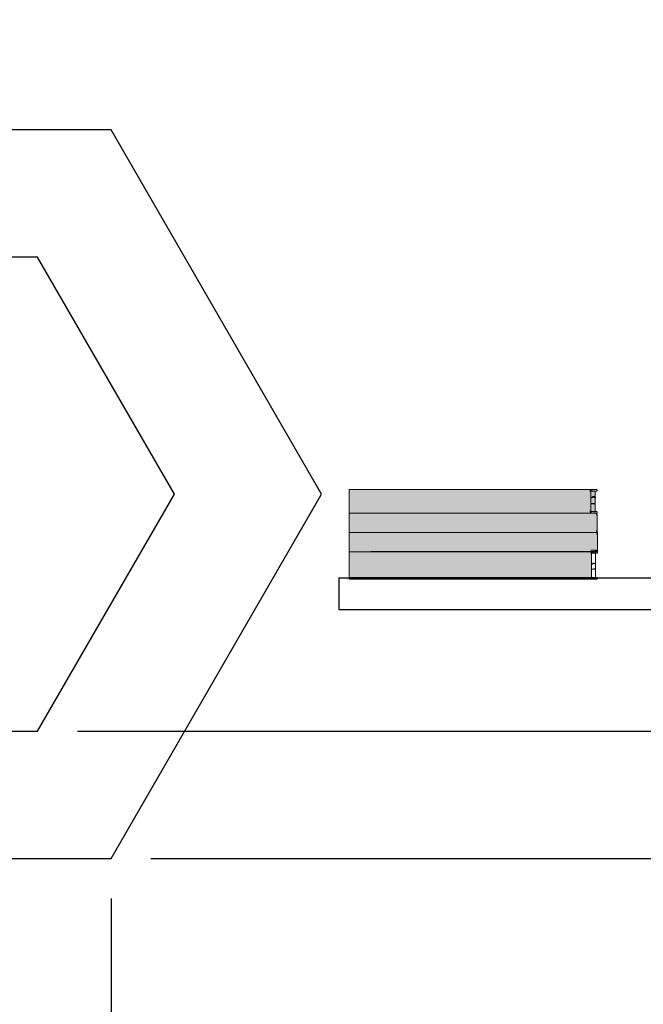
# Model space of a CAD drawing. Units: millimetres. Extents: x 7894 to 8038, y 6851 to 6951.
# Tile 24 of 49: x 7948.9 to 7958.7, y 6916.43 to 6931.89. Entities that reach past the tile are written whole.
import ezdxf

# ---------------------------------------------------------------- set-up
doc = ezdxf.new("R2010")
doc.units = ezdxf.units.MM
for name, color, linetype, lineweight in [('A-ANNO-DIMS', 2, 'Continuous', 18), ('A-FURN-BOOK', 8, 'Continuous', 13), ('A-FURN-CASE', 7, 'Continuous', 30), ('A-FURN-SHLF', 7, 'Continuous', 30)]:
    doc.layers.add(name, color=color, linetype=linetype, lineweight=lineweight)
doc.layers.add('A-FURN-PATT', color=32, linetype='Continuous', lineweight=9, true_color=0xcd6928)
doc.styles.get("Standard").update_dxf_attribs({"font": 'arial.ttf'})
doc.dimstyles.new('ISO-25', dxfattribs={"dimtxt": 1, "dimasz": 1, "dimexe": 1.25, "dimexo": 0.625, "dimtad": 1, "dimdec": 0, "dimlunit": 4, "dimtxsty": 'Standard', "dimcen": 2.5, "dimclrt": 1, "dimadec": 0, "dimazin": 0, "dimtfac": 1, "dimtdec": 0, "dimtmove": 0, "dimatfit": 3, "dimfxl": 1, "dimarcsym": 0})

# ---------------------------------------------------------------- blocks, each defined once
blk = doc.blocks.new('*D23')
at = {"layer": 'A-ANNO-DIMS', "color": 0, "lineweight": -2, "transparency": 16777216}
for p, q in [((7940.089, 6907.098), (7940.089, 6947.793)), ((7971.936, 6928.989), (7971.936, 6947.793)), ((7941.089, 6946.543), (7970.936, 6946.543))]:
    blk.add_line(p, q, dxfattribs=at)
at = {"layer": 'A-ANNO-DIMS', "color": 0, "transparency": 16777216}
for points in [[(7941.089, 6946.709), (7941.089, 6946.376), (7940.089, 6946.543)], [(7970.936, 6946.709), (7970.936, 6946.376), (7971.936, 6946.543)]]:
    blk.add_solid(points, dxfattribs=at)
at = {"layer": 'Defpoints', "color": 0, "transparency": 16777216}
for p in [(7971.936, 6946.543), (7971.936, 6928.364), (7940.089, 6906.473)]:
    blk.add_point(p, dxfattribs=at)
at = {"layer": 'A-ANNO-DIMS', "color": 1, "transparency": 16777216, "insert": (7956.012, 6947.678), "char_height": 1, "attachment_point": 5}
blk.add_mtext('2\'-8"', dxfattribs=at)
blk = doc.blocks.new('*D24')
at = {"layer": 'A-ANNO-DIMS', "color": 0, "lineweight": -2, "transparency": 16777216}
for p, q in [((7953.341, 6944.606), (7936.902, 6944.606)), ((7938.152, 6907.473), (7938.152, 6943.606)), ((7939.464, 6906.473), (7936.902, 6906.473))]:
    blk.add_line(p, q, dxfattribs=at)
at = {"layer": 'A-ANNO-DIMS', "color": 0, "transparency": 16777216}
for points in [[(7937.986, 6943.606), (7938.319, 6943.606), (7938.152, 6944.606)], [(7937.986, 6907.473), (7938.319, 6907.473), (7938.152, 6906.473)]]:
    blk.add_solid(points, dxfattribs=at)
at = {"layer": 'Defpoints', "color": 0, "transparency": 16777216}
for p in [(7938.152, 6944.606), (7953.966, 6944.606), (7940.089, 6906.473)]:
    blk.add_point(p, dxfattribs=at)
at = {"layer": 'A-ANNO-DIMS', "color": 1, "transparency": 16777216, "insert": (7937.016, 6925.539), "char_height": 1, "attachment_point": 5, "rotation": 90}
blk.add_mtext('3\'-2"', dxfattribs=at)
blk = doc.blocks.new('*D26')
at = {"layer": 'A-ANNO-DIMS', "color": 0, "lineweight": -2, "transparency": 16777216}
for p, q in [((7950.965, 6918.72), (7975.227, 6918.72)), ((7973.977, 6917.72), (7973.977, 6907.473)), ((7964.966, 6906.473), (7975.227, 6906.473))]:
    blk.add_line(p, q, dxfattribs=at)
at = {"layer": 'A-ANNO-DIMS', "color": 0, "transparency": 16777216}
for points in [[(7973.811, 6917.72), (7974.144, 6917.72), (7973.977, 6918.72)], [(7973.811, 6907.473), (7974.144, 6907.473), (7973.977, 6906.473)]]:
    blk.add_solid(points, dxfattribs=at)
at = {"layer": 'Defpoints', "color": 0, "transparency": 16777216}
for p in [(7950.34, 6918.72), (7964.341, 6906.473), (7973.977, 6906.473)]:
    blk.add_point(p, dxfattribs=at)
at = {"layer": 'A-ANNO-DIMS', "color": 1, "transparency": 16777216, "insert": (7972.842, 6912.597), "char_height": 1, "attachment_point": 5, "rotation": 90}
blk.add_mtext('1\'-0"', dxfattribs=at)
blk = doc.blocks.new('*D27')
at = {"layer": 'A-ANNO-DIMS', "color": 0, "lineweight": -2, "transparency": 16777216}
for p, q in [((7971.842, 6922.628), (7975.227, 6922.628)), ((7973.977, 6921.628), (7973.977, 6919.72)), ((7950.965, 6918.72), (7975.227, 6918.72))]:
    blk.add_line(p, q, dxfattribs=at)
at = {"layer": 'A-ANNO-DIMS', "color": 0, "transparency": 16777216}
for points in [[(7973.811, 6921.628), (7974.144, 6921.628), (7973.977, 6922.628)], [(7973.811, 6919.72), (7974.144, 6919.72), (7973.977, 6918.72)]]:
    blk.add_solid(points, dxfattribs=at)
at = {"layer": 'Defpoints', "color": 0, "transparency": 16777216}
for p in [(7971.217, 6922.628), (7950.34, 6918.72), (7973.977, 6918.72)]:
    blk.add_point(p, dxfattribs=at)
at = {"layer": 'A-ANNO-DIMS', "color": 1, "transparency": 16777216, "insert": (7972.842, 6920.674), "char_height": 1, "attachment_point": 5, "rotation": 90}
blk.add_mtext('0\'-4"', dxfattribs=at)
blk = doc.blocks.new('*D29')
at = {"layer": 'A-ANNO-DIMS', "color": 0, "lineweight": -2, "transparency": 16777216}
for p, q in [((7940.435, 6923.814), (7940.435, 6903.287)), ((7943.737, 6918.095), (7943.737, 6903.287)), ((7941.435, 6904.537), (7942.737, 6904.537)), ((7943.737, 6904.537), (7950.975, 6904.537))]:
    blk.add_line(p, q, dxfattribs=at)
at = {"layer": 'A-ANNO-DIMS', "color": 0, "transparency": 16777216}
for points in [[(7941.435, 6904.703), (7941.435, 6904.37), (7940.435, 6904.537)], [(7942.737, 6904.703), (7942.737, 6904.37), (7943.737, 6904.537)]]:
    blk.add_solid(points, dxfattribs=at)
at = {"layer": 'Defpoints', "color": 0, "transparency": 16777216}
for p in [(7940.435, 6924.439), (7943.737, 6918.72), (7943.737, 6904.537)]:
    blk.add_point(p, dxfattribs=at)
at = {"layer": 'A-ANNO-DIMS', "color": 1, "transparency": 16777216, "insert": (7947.856, 6905.679), "char_height": 1, "attachment_point": 5}
blk.add_mtext('0\'-3 1/2"', dxfattribs=at)
blk = doc.blocks.new('*D31')
at = {"layer": 'A-ANNO-DIMS', "color": 0, "lineweight": -2, "transparency": 16777216}
for p, q in [((7973.977, 6921.72), (7973.977, 6926.628)), ((7949.811, 6920.72), (7975.227, 6920.72)), ((7973.977, 6918.72), (7973.977, 6920.72)), ((7950.965, 6918.72), (7975.227, 6918.72)), ((7973.977, 6917.72), (7973.977, 6916.72))]:
    blk.add_line(p, q, dxfattribs=at)
at = {"layer": 'A-ANNO-DIMS', "color": 0, "transparency": 16777216}
for points in [[(7973.811, 6921.72), (7974.144, 6921.72), (7973.977, 6920.72)], [(7973.811, 6917.72), (7974.144, 6917.72), (7973.977, 6918.72)]]:
    blk.add_solid(points, dxfattribs=at)
at = {"layer": 'Defpoints', "color": 0, "transparency": 16777216}
for p in [(7949.186, 6920.72), (7973.977, 6920.72), (7950.34, 6918.72)]:
    blk.add_point(p, dxfattribs=at)
at = {"layer": 'A-ANNO-DIMS', "color": 1, "transparency": 16777216, "insert": (7972.842, 6924.674), "char_height": 1, "attachment_point": 5, "rotation": 90}
blk.add_mtext('0\'-2"', dxfattribs=at)
blk = doc.blocks.new('*D32')
at = {"layer": 'A-ANNO-DIMS', "color": 0, "lineweight": -2, "transparency": 16777216}
for p, q in [((7943.737, 6918.095), (7943.737, 6903.287)), ((7950.34, 6918.095), (7950.34, 6903.287)), ((7944.737, 6904.537), (7949.34, 6904.537))]:
    blk.add_line(p, q, dxfattribs=at)
at = {"layer": 'A-ANNO-DIMS', "color": 0, "transparency": 16777216}
for points in [[(7944.737, 6904.703), (7944.737, 6904.37), (7943.737, 6904.537)], [(7949.34, 6904.703), (7949.34, 6904.37), (7950.34, 6904.537)]]:
    blk.add_solid(points, dxfattribs=at)
at = {"layer": 'Defpoints', "color": 0, "transparency": 16777216}
for p in [(7943.737, 6918.72), (7950.34, 6918.72), (7950.34, 6904.537)]:
    blk.add_point(p, dxfattribs=at)
at = {"layer": 'A-ANNO-DIMS', "color": 1, "transparency": 16777216, "insert": (7947.038, 6905.679), "char_height": 1, "attachment_point": 5}
blk.add_mtext('0\'-6 1/2"', dxfattribs=at)

msp = doc.modelspace()

# ---------------------------------------------------------------- hatches: boundary and pattern name
at = {"layer": 'A-FURN-PATT'}
h = msp.add_hatch(color=256, dxfattribs=at)
h.dxf.hatch_style = 1
h.paths.add_polyline_path([(7957.95, 6924.386), (7957.938, 6924.384), (7957.938, 6924.363), (7957.938, 6924.29), (7957.938, 6924.243), (7957.939, 6924.2), (7957.939, 6924.165), (7957.971, 6924.165), (7957.971, 6924.134), (7957.972, 6924.133), (7957.972, 6924.132), (7957.972, 6924.132), (7957.972, 6924.121), (7957.972, 6924.119), (7957.972, 6924.119), (7957.972, 6924.118), (7957.972, 6923.837), (7957.979, 6923.832), (7957.979, 6923.819), (7957.978, 6923.818), (7957.978, 6923.818), (7957.978, 6923.817), (7957.977, 6923.814), (7957.977, 6923.812), (7957.976, 6923.811), (7957.973, 6923.813), (7957.977, 6923.817), (7957.976, 6923.828), (7957.976, 6923.831), (7957.968, 6923.838), (7954.076, 6923.838), (7954.076, 6924.511), (7957.866, 6924.511), (7957.971, 6924.511), (7957.971, 6924.486), (7957.939, 6924.486), (7957.939, 6924.453), (7957.938, 6924.393)])
h.paths.add_polyline_path([(7957.874, 6924.165), (7957.874, 6924.166), (7957.874, 6924.166), (7957.873, 6924.166)], flags=16)
h.paths.add_polyline_path([(7957.865, 6924.139), (7957.873, 6924.145), (7957.874, 6924.146), (7957.875, 6924.154), (7957.863, 6924.154), (7957.854, 6924.165), (7957.874, 6924.165), (7957.874, 6924.167), (7957.876, 6924.165), (7957.878, 6924.165), (7957.876, 6924.165), (7957.876, 6924.165), (7957.876, 6924.163), (7957.876, 6924.16), (7957.877, 6924.158), (7957.875, 6924.159), (7957.874, 6924.152), (7957.873, 6924.14), (7957.963, 6924.14), (7957.965, 6924.139)], flags=16)
h.paths.add_polyline_path([(7957.874, 6924.49), (7957.874, 6924.489), (7957.874, 6924.49)], flags=16)
h.paths.add_polyline_path([(7957.873, 6924.491), (7957.874, 6924.491), (7957.874, 6924.496), (7957.868, 6924.496)], flags=16)
h.paths.add_polyline_path([(7957.874, 6924.483), (7957.874, 6924.441), (7957.873, 6924.388), (7957.873, 6924.388), (7957.883, 6924.388), (7957.908, 6924.403), (7957.924, 6924.401), (7957.918, 6924.398), (7957.932, 6924.391), (7957.938, 6924.384), (7957.935, 6924.386), (7957.931, 6924.388), (7957.915, 6924.396), (7957.897, 6924.386), (7957.882, 6924.384), (7957.881, 6924.384), (7957.873, 6924.384), (7957.873, 6924.384), (7957.874, 6924.441), (7957.874, 6924.483), (7957.868, 6924.478), (7957.865, 6924.478), (7957.854, 6924.486), (7957.865, 6924.486), (7957.879, 6924.486), (7957.878, 6924.487)], flags=16)
h.paths.add_polyline_path([(7957.875, 6924.492), (7957.874, 6924.504), (7957.866, 6924.511), (7957.873, 6924.511), (7957.875, 6924.492), (7957.875, 6924.492)], flags=16)
h.paths.add_polyline_path([(7957.884, 6924.386), (7957.873, 6924.386), (7957.873, 6924.384), (7957.876, 6924.381)], flags=16)
h.paths.add_polyline_path([(7957.873, 6924.386), (7957.873, 6924.386), (7957.873, 6924.384), (7957.873, 6924.386)], flags=0)
h.paths.add_polyline_path([(7957.918, 6924.398), (7957.914, 6924.4), (7957.908, 6924.4), (7957.915, 6924.396)], flags=0)
h = msp.add_hatch(color=256, dxfattribs=at)
h.dxf.hatch_style = 1
h.paths.add_polyline_path([(7957.979, 6923.654), (7957.979, 6923.719), (7957.979, 6923.776), (7957.979, 6923.816), (7957.977, 6923.817), (7957.977, 6923.817), (7957.979, 6923.817), (7957.979, 6923.823), (7957.979, 6923.832), (7957.971, 6923.838), (7957.968, 6923.838), (7954.076, 6923.838), (7954.076, 6923.537), (7957.874, 6923.537), (7957.968, 6923.538), (7957.969, 6923.538), (7957.969, 6923.538), (7957.971, 6923.538), (7957.979, 6923.544), (7957.978, 6923.558), (7957.978, 6923.559), (7957.978, 6923.559), (7957.977, 6923.563), (7957.979, 6923.561), (7957.979, 6923.565)])
h = msp.add_hatch(color=256, dxfattribs=at)
h.dxf.hatch_style = 1
h.paths.add_polyline_path([(7957.88, 6923.348), (7957.88, 6923.352), (7957.881, 6923.367), (7957.881, 6923.451), (7957.88, 6923.466), (7957.881, 6923.504), (7957.881, 6923.511), (7957.88, 6923.512), (7957.88, 6923.512), (7957.881, 6923.517), (7957.881, 6923.517), (7957.881, 6923.517), (7957.88, 6923.518), (7957.881, 6923.518), (7957.882, 6923.525), (7957.881, 6923.53), (7957.877, 6923.534), (7957.874, 6923.537), (7954.076, 6923.537), (7954.076, 6923.132), (7957.832, 6923.132), (7957.873, 6923.132), (7957.881, 6923.132), (7957.881, 6923.134), (7957.881, 6923.141), (7957.88, 6923.179), (7957.881, 6923.191), (7957.88, 6923.265), (7957.88, 6923.267), (7957.881, 6923.27)])
h.paths.add_polyline_path([(7957.881, 6923.531), (7957.881, 6923.531), (7957.881, 6923.53)], flags=17)

# ---------------------------------------------------------------- linework, layer by layer
at = {"layer": 'A-FURN-BOOK'}
for p, q in [((7957.866, 6924.511, 2.152), (7954.076, 6924.511, 2.152)), ((7954.076, 6923.108, 2.152), (7954.076, 6924.511, 2.152)), ((7957.868, 6924.496, 2.152), (7957.854, 6924.496, 2.152)), ((7957.855, 6924.491, 2.152), (7957.854, 6924.492, 2.152)), ((7957.854, 6924.486, 2.152), (7957.865, 6924.486, 2.152)), ((7957.856, 6924.478, 2.152), (7957.854, 6924.478, 2.152)), ((7957.855, 6924.453, 2.152), (7957.854, 6924.453, 2.152)), ((7957.87, 6924.492, 2.152), (7957.855, 6924.491, 2.152)), ((7957.866, 6924.484, 2.152), (7957.865, 6924.484, 2.152)), ((7957.868, 6924.478, 2.152), (7957.865, 6924.478, 2.152)), ((7957.869, 6924.508, 2.152), (7957.866, 6924.511, 2.152)), ((7957.963, 6924.511, 2.152), (7957.866, 6924.511, 2.152)), ((7957.867, 6924.485, 2.152), (7957.866, 6924.484, 2.152)), ((7957.871, 6924.493, 2.152), (7957.868, 6924.496, 2.152)), ((7957.874, 6924.483, 2.152), (7957.868, 6924.478, 2.152)), ((7957.869, 6924.508, 2.152), (7957.873, 6924.505, 2.152)), ((7957.873, 6924.504, 2.152), (7957.873, 6924.505, 2.152)), ((7957.874, 6924.491, 2.152), (7957.873, 6924.491, 2.152)), ((7957.873, 6924.491, 2.152), (7957.874, 6924.491, 2.152)), ((7957.874, 6924.49, 2.152), (7957.873, 6924.49, 2.152)), ((7957.873, 6924.486, 2.152), (7957.874, 6924.49, 2.152)), ((7957.874, 6924.485, 2.152), (7957.873, 6924.486, 2.152)), ((7957.874, 6924.486, 2.152), (7957.873, 6924.486, 2.152)), ((7957.873, 6924.388, 2.152), (7957.874, 6924.441, 2.152)), ((7957.874, 6924.498, 2.152), (7957.874, 6924.504, 2.152)), ((7957.874, 6924.504, 2.152), (7957.873, 6924.504, 2.152)), ((7957.875, 6924.492, 2.152), (7957.874, 6924.498, 2.152)), ((7957.874, 6924.491, 2.152), (7957.874, 6924.498, 2.152)), ((7957.874, 6924.491, 2.152), (7957.875, 6924.492, 2.152)), ((7957.875, 6924.489, 2.152), (7957.874, 6924.491, 2.152)), ((7957.874, 6924.49, 2.152), (7957.874, 6924.491, 2.152)), ((7957.874, 6924.491, 2.152), (7957.874, 6924.491, 2.152)), ((7957.875, 6924.485, 2.152), (7957.874, 6924.486, 2.152)), ((7957.874, 6924.483, 2.152), (7957.874, 6924.485, 2.152)), ((7957.875, 6924.485, 2.152), (7957.874, 6924.483, 2.152)), ((7957.874, 6924.477, 2.152), (7957.874, 6924.483, 2.152)), ((7957.874, 6924.441, 2.152), (7957.874, 6924.477, 2.152)), ((7957.877, 6924.493, 2.152), (7957.875, 6924.492, 2.152)), ((7957.875, 6924.492, 2.152), (7957.876, 6924.491, 2.152)), ((7957.875, 6924.489, 2.152), (7957.875, 6924.492, 2.152)), ((7957.875, 6924.485, 2.152), (7957.876, 6924.487, 2.152)), ((7957.875, 6924.485, 2.152), (7957.878, 6924.486, 2.152)), ((7957.875, 6924.485, 2.152), (7957.875, 6924.485, 2.152)), ((7957.876, 6924.491, 2.152), (7957.877, 6924.493, 2.152)), ((7957.876, 6924.491, 2.152), (7957.878, 6924.492, 2.152)), ((7957.876, 6924.487, 2.152), (7957.876, 6924.491, 2.152)), ((7957.876, 6924.491, 2.152), (7957.876, 6924.491, 2.152)), ((7957.878, 6924.486, 2.152), (7957.939, 6924.486, 2.152)), ((7957.882, 6924.491, 2.152), (7957.88, 6924.492, 2.152)), ((7957.896, 6924.492, 2.152), (7957.882, 6924.491, 2.152)), ((7957.939, 6924.453, 2.152), (7957.938, 6924.41, 2.152)), ((7957.939, 6924.486, 2.152), (7957.939, 6924.453, 2.152)), ((7957.939, 6924.486, 2.152), (7957.963, 6924.486, 2.152)), ((7957.963, 6924.511, 2.152), (7957.971, 6924.504, 2.152)), ((7957.971, 6924.493, 2.152), (7957.963, 6924.486, 2.152)), ((7957.971, 6924.504, 2.152), (7957.971, 6924.493, 2.152)), ((7957.873, 6924.388, 2.152), (7957.873, 6924.388, 2.152)), ((7957.873, 6924.388, 2.152), (7957.873, 6924.388, 2.152)), ((7957.873, 6924.386, 2.152), (7957.873, 6924.388, 2.152)), ((7957.873, 6924.388, 2.152), (7957.873, 6924.388, 2.152)), ((7957.873, 6924.386, 2.152), (7957.873, 6924.386, 2.152)), ((7957.873, 6924.384, 2.152), (7957.873, 6924.386, 2.152)), ((7957.873, 6924.386, 2.152), (7957.873, 6924.386, 2.152)), ((7957.873, 6924.386, 2.152), (7957.884, 6924.386, 2.152)), ((7957.873, 6924.384, 2.152), (7957.873, 6924.384, 2.152)), ((7957.873, 6924.384, 2.152), (7957.873, 6924.384, 2.152)), ((7957.873, 6924.365, 2.152), (7957.873, 6924.384, 2.152)), ((7957.873, 6924.384, 2.152), (7957.873, 6924.384, 2.152)), ((7957.873, 6924.292, 2.152), (7957.873, 6924.365, 2.152)), ((7957.873, 6924.288, 2.152), (7957.873, 6924.292, 2.152)), ((7957.873, 6924.292, 2.152), (7957.881, 6924.292, 2.152)), ((7957.873, 6924.28, 2.152), (7957.873, 6924.288, 2.152)), ((7957.873, 6924.288, 2.152), (7957.873, 6924.288, 2.152)), ((7957.873, 6924.288, 2.152), (7957.881, 6924.288, 2.152)), ((7957.873, 6924.28, 2.152), (7957.874, 6924.174, 2.152)), ((7957.881, 6924.388, 2.152), (7957.873, 6924.388, 2.152)), ((7957.873, 6924.386, 2.152), (7957.884, 6924.386, 2.152)), ((7957.881, 6924.384, 2.152), (7957.873, 6924.384, 2.152)), ((7957.881, 6924.388, 2.152), (7957.882, 6924.388, 2.152)), ((7957.881, 6924.388, 2.152), (7957.881, 6924.388, 2.152)), ((7957.882, 6924.384, 2.152), (7957.881, 6924.384, 2.152)), ((7957.881, 6924.292, 2.152), (7957.938, 6924.292, 2.152)), ((7957.881, 6924.288, 2.152), (7957.938, 6924.288, 2.152)), ((7957.883, 6924.388, 2.152), (7957.882, 6924.388, 2.152)), ((7957.897, 6924.386, 2.152), (7957.882, 6924.384, 2.152)), ((7957.884, 6924.386, 2.152), (7957.882, 6924.384, 2.152)), ((7957.883, 6924.388, 2.152), (7957.908, 6924.403, 2.152)), ((7957.884, 6924.386, 2.152), (7957.885, 6924.386, 2.152)), ((7957.897, 6924.386, 2.152), (7957.885, 6924.386, 2.152)), ((7957.908, 6924.4, 2.152), (7957.896, 6924.393, 2.152)), ((7957.897, 6924.386, 2.152), (7957.915, 6924.396, 2.152)), ((7957.924, 6924.401, 2.152), (7957.908, 6924.403, 2.152)), ((7957.908, 6924.403, 2.152), (7957.914, 6924.4, 2.152)), ((7957.912, 6924.398, 2.152), (7957.908, 6924.4, 2.152)), ((7957.914, 6924.4, 2.152), (7957.908, 6924.4, 2.152)), ((7957.924, 6924.401, 2.152), (7957.914, 6924.4, 2.152)), ((7957.914, 6924.4, 2.152), (7957.917, 6924.399, 2.152)), ((7957.938, 6924.292, 2.152), (7957.914, 6924.29, 2.152)), ((7957.914, 6924.29, 2.152), (7957.938, 6924.288, 2.152)), ((7957.915, 6924.396, 2.152), (7957.918, 6924.398, 2.152)), ((7957.931, 6924.388, 2.152), (7957.915, 6924.396, 2.152)), ((7957.918, 6924.398, 2.152), (7957.924, 6924.401, 2.152)), ((7957.918, 6924.398, 2.152), (7957.932, 6924.391, 2.152)), ((7957.938, 6924.393, 2.152), (7957.924, 6924.401, 2.152)), ((7957.935, 6924.388, 2.152), (7957.931, 6924.388, 2.152)), ((7957.935, 6924.386, 2.152), (7957.931, 6924.388, 2.152)), ((7957.935, 6924.386, 2.152), (7957.937, 6924.386, 2.152)), ((7957.938, 6924.384, 2.152), (7957.935, 6924.386, 2.152)), ((7957.938, 6924.41, 2.152), (7957.938, 6924.393, 2.152)), ((7957.95, 6924.386, 2.152), (7957.938, 6924.393, 2.152)), ((7957.95, 6924.386, 2.152), (7957.938, 6924.384, 2.152)), ((7957.938, 6924.384, 2.152), (7957.938, 6924.363, 2.152)), ((7957.938, 6924.292, 2.152), (7957.938, 6924.363, 2.152)), ((7957.938, 6924.243, 2.152), (7957.938, 6924.288, 2.152)), ((7957.866, 6924.14, 2.152), (7954.076, 6924.14, 2.152)), ((7957.965, 6924.139, 2.152), (7954.165, 6924.139, 2.152)), ((7957.854, 6924.2, 2.152), (7957.855, 6924.2, 2.152)), ((7957.863, 6924.173, 2.152), (7957.854, 6924.173, 2.152)), ((7957.865, 6924.166, 2.152), (7957.854, 6924.166, 2.152)), ((7957.854, 6924.165, 2.152), (7957.868, 6924.165, 2.152)), ((7957.87, 6924.161, 2.152), (7957.857, 6924.161, 2.152)), ((7957.857, 6924.161, 2.152), (7957.87, 6924.161, 2.152)), ((7957.867, 6924.154, 2.152), (7957.863, 6924.154, 2.152)), ((7957.866, 6924.14, 2.152), (7957.873, 6924.145, 2.152)), ((7957.866, 6924.14, 2.152), (7957.963, 6924.14, 2.152)), ((7957.868, 6924.165, 2.152), (7957.867, 6924.165, 2.152)), ((7957.869, 6924.165, 2.152), (7957.868, 6924.165, 2.152)), ((7957.869, 6924.165, 2.152), (7957.871, 6924.163, 2.152)), ((7957.871, 6924.163, 2.152), (7957.869, 6924.165, 2.152)), ((7957.872, 6924.165, 2.152), (7957.869, 6924.165, 2.152)), ((7957.874, 6924.167, 2.152), (7957.873, 6924.168, 2.152)), ((7957.873, 6924.165, 2.152), (7957.874, 6924.166, 2.152)), ((7957.874, 6924.165, 2.152), (7957.873, 6924.165, 2.152)), ((7957.873, 6924.161, 2.152), (7957.873, 6924.165, 2.152)), ((7957.874, 6924.161, 2.152), (7957.873, 6924.161, 2.152)), ((7957.873, 6924.161, 2.152), (7957.874, 6924.161, 2.152)), ((7957.874, 6924.16, 2.152), (7957.873, 6924.159, 2.152)), ((7957.873, 6924.145, 2.152), (7957.874, 6924.146, 2.152)), ((7957.874, 6924.167, 2.152), (7957.874, 6924.174, 2.152)), ((7957.874, 6924.166, 2.152), (7957.874, 6924.167, 2.152)), ((7957.875, 6924.166, 2.152), (7957.874, 6924.167, 2.152)), ((7957.875, 6924.165, 2.152), (7957.874, 6924.165, 2.152)), ((7957.874, 6924.16, 2.152), (7957.874, 6924.161, 2.152)), ((7957.875, 6924.161, 2.152), (7957.874, 6924.16, 2.152)), ((7957.875, 6924.161, 2.152), (7957.874, 6924.161, 2.152)), ((7957.874, 6924.16, 2.152), (7957.874, 6924.16, 2.152)), ((7957.874, 6924.16, 2.152), (7957.874, 6924.152, 2.152)), ((7957.874, 6924.16, 2.152), (7957.875, 6924.159, 2.152)), ((7957.874, 6924.152, 2.152), (7957.875, 6924.159, 2.152)), ((7957.874, 6924.146, 2.152), (7957.874, 6924.152, 2.152)), ((7957.875, 6924.165, 2.152), (7957.875, 6924.166, 2.152)), ((7957.878, 6924.165, 2.152), (7957.875, 6924.165, 2.152)), ((7957.876, 6924.163, 2.152), (7957.875, 6924.165, 2.152)), ((7957.875, 6924.159, 2.152), (7957.875, 6924.161, 2.152)), ((7957.875, 6924.159, 2.152), (7957.877, 6924.158, 2.152)), ((7957.876, 6924.16, 2.152), (7957.876, 6924.163, 2.152)), ((7957.877, 6924.158, 2.152), (7957.876, 6924.16, 2.152)), ((7957.939, 6924.165, 2.152), (7957.878, 6924.165, 2.152)), ((7957.939, 6924.161, 2.152), (7957.92, 6924.161, 2.152)), ((7957.92, 6924.161, 2.152), (7957.92, 6924.161, 2.152)), ((7957.938, 6924.243, 2.152), (7957.939, 6924.2, 2.152)), ((7957.939, 6924.2, 2.152), (7957.939, 6924.165, 2.152)), ((7957.939, 6924.165, 2.152), (7957.939, 6924.161, 2.152)), ((7957.939, 6924.165, 2.152), (7957.963, 6924.165, 2.152)), ((7957.965, 6924.125, 2.152), (7957.956, 6924.125, 2.152)), ((7957.963, 6924.165, 2.152), (7957.971, 6924.158, 2.152)), ((7957.971, 6924.147, 2.152), (7957.963, 6924.14, 2.152)), ((7957.965, 6924.139, 2.152), (7957.972, 6924.132, 2.152)), ((7957.972, 6924.132, 2.152), (7957.965, 6924.139, 2.152)), ((7957.965, 6924.139, 2.152), (7957.972, 6924.133, 2.152)), ((7957.97, 6924.12, 2.152), (7957.965, 6924.125, 2.152)), ((7957.97, 6924.12, 2.152), (7957.965, 6924.114, 2.152)), ((7957.972, 6924.118, 2.152), (7957.965, 6924.113, 2.152)), ((7957.972, 6924.121, 2.152), (7957.97, 6924.12, 2.152)), ((7957.972, 6924.118, 2.152), (7957.97, 6924.12, 2.152)), ((7957.971, 6924.158, 2.152), (7957.971, 6924.147, 2.152)), ((7957.972, 6924.132, 2.152), (7957.972, 6924.133, 2.152)), ((7957.972, 6924.132, 2.152), (7957.972, 6924.132, 2.152)), ((7957.972, 6924.121, 2.152), (7957.972, 6924.132, 2.152)), ((7957.972, 6924.119, 2.152), (7957.972, 6924.121, 2.152)), ((7957.972, 6924.119, 2.152), (7957.972, 6924.118, 2.152)), ((7957.972, 6924.118, 2.152), (7957.972, 6924.119, 2.152)), ((7957.972, 6924.118, 2.152), (7957.972, 6924.119, 2.152)), ((7957.972, 6924.119, 2.152), (7957.972, 6924.119, 2.152)), ((7957.972, 6924.119, 2.152), (7957.972, 6924.118, 2.152)), ((7957.972, 6924.118, 2.152), (7957.972, 6924.118, 2.152)), ((7957.972, 6924.118, 2.152), (7957.972, 6924.118, 2.152)), ((7957.972, 6924.113, 2.152), (7957.972, 6924.118, 2.152)), ((7957.972, 6924.113, 2.152), (7957.965, 6924.107, 2.152)), ((7957.972, 6924.113, 2.152), (7957.972, 6923.845, 2.152)), ((7957.965, 6923.839, 2.152), (7954.076, 6923.839, 2.152)), ((7954.076, 6923.838, 2.152), (7957.968, 6923.838, 2.152)), ((7957.953, 6923.863, 2.152), (7957.965, 6923.863, 2.152)), ((7957.963, 6923.824, 2.152), (7957.96, 6923.824, 2.152)), ((7957.968, 6923.813, 2.152), (7957.961, 6923.813, 2.152)), ((7957.965, 6923.853, 2.152), (7957.962, 6923.853, 2.152)), ((7957.966, 6923.87, 2.152), (7957.965, 6923.871, 2.152)), ((7957.965, 6923.863, 2.152), (7957.969, 6923.859, 2.152)), ((7957.967, 6923.855, 2.152), (7957.965, 6923.853, 2.152)), ((7957.972, 6923.845, 2.152), (7957.965, 6923.839, 2.152)), ((7957.97, 6923.861, 2.152), (7957.966, 6923.864, 2.152)), ((7957.968, 6923.838, 2.152), (7957.971, 6923.835, 2.152)), ((7957.971, 6923.838, 2.152), (7957.968, 6923.838, 2.152)), ((7957.972, 6923.865, 2.152), (7957.971, 6923.866, 2.152)), ((7957.971, 6923.838, 2.152), (7957.979, 6923.832, 2.152)), ((7957.973, 6923.813, 2.152), (7957.972, 6923.813, 2.152)), ((7957.973, 6923.813, 2.152), (7957.977, 6923.817, 2.152)), ((7957.976, 6923.83, 2.152), (7957.976, 6923.828, 2.152)), ((7957.976, 6923.828, 2.152), (7957.976, 6923.824, 2.152)), ((7957.977, 6923.817, 2.152), (7957.976, 6923.818, 2.152)), ((7957.977, 6923.812, 2.152), (7957.976, 6923.811, 2.152)), ((7957.977, 6923.819, 2.152), (7957.977, 6923.817, 2.152)), ((7957.977, 6923.817, 2.152), (7957.977, 6923.817, 2.152)), ((7957.978, 6923.817, 2.152), (7957.977, 6923.814, 2.152)), ((7957.977, 6923.817, 2.152), (7957.978, 6923.817, 2.152)), ((7957.977, 6923.814, 2.152), (7957.977, 6923.812, 2.152)), ((7957.978, 6923.818, 2.152), (7957.978, 6923.822, 2.152)), ((7957.978, 6923.818, 2.152), (7957.978, 6923.817, 2.152)), ((7957.979, 6923.832, 2.152), (7957.979, 6923.823, 2.152)), ((7957.979, 6923.823, 2.152), (7957.979, 6923.832, 2.152)), ((7957.979, 6923.823, 2.152), (7957.979, 6923.776, 2.152)), ((7957.979, 6923.776, 2.152), (7957.979, 6923.719, 2.152)), ((7957.979, 6923.719, 2.152), (7957.979, 6923.654, 2.152)), ((7957.979, 6923.654, 2.152), (7957.979, 6923.565, 2.152)), ((7954.076, 6923.537, 2.152), (7957.874, 6923.537, 2.152)), ((7957.971, 6923.538, 2.152), (7954.42, 6923.538, 2.152)), ((7957.931, 6923.562, 2.152), (7957.872, 6923.562, 2.152)), ((7957.875, 6923.523, 2.152), (7957.873, 6923.523, 2.152)), ((7957.877, 6923.518, 2.152), (7957.873, 6923.518, 2.152)), ((7957.874, 6923.511, 2.152), (7957.873, 6923.511, 2.152)), ((7957.875, 6923.505, 2.152), (7957.873, 6923.505, 2.152)), ((7957.877, 6923.534, 2.152), (7957.874, 6923.537, 2.152)), ((7957.874, 6923.537, 2.152), (7957.97, 6923.537, 2.152)), ((7957.874, 6923.512, 2.152), (7957.874, 6923.511, 2.152)), ((7957.879, 6923.52, 2.152), (7957.875, 6923.523, 2.152)), ((7957.881, 6923.51, 2.152), (7957.875, 6923.505, 2.152)), ((7957.88, 6923.531, 2.152), (7957.877, 6923.534, 2.152)), ((7957.877, 6923.534, 2.152), (7957.881, 6923.531, 2.152)), ((7957.881, 6923.517, 2.152), (7957.88, 6923.518, 2.152)), ((7957.881, 6923.518, 2.152), (7957.88, 6923.518, 2.152)), ((7957.881, 6923.517, 2.152), (7957.88, 6923.516, 2.152)), ((7957.88, 6923.512, 2.152), (7957.881, 6923.517, 2.152)), ((7957.881, 6923.511, 2.152), (7957.88, 6923.512, 2.152)), ((7957.881, 6923.512, 2.152), (7957.88, 6923.512, 2.152)), ((7957.88, 6923.466, 2.152), (7957.881, 6923.504, 2.152)), ((7957.881, 6923.53, 2.152), (7957.881, 6923.531, 2.152)), ((7957.881, 6923.53, 2.152), (7957.881, 6923.531, 2.152)), ((7957.881, 6923.531, 2.152), (7957.881, 6923.531, 2.152)), ((7957.882, 6923.525, 2.152), (7957.881, 6923.53, 2.152)), ((7957.881, 6923.518, 2.152), (7957.882, 6923.525, 2.152)), ((7957.881, 6923.518, 2.152), (7957.881, 6923.517, 2.152)), ((7957.882, 6923.518, 2.152), (7957.881, 6923.518, 2.152)), ((7957.883, 6923.516, 2.152), (7957.881, 6923.517, 2.152)), ((7957.881, 6923.517, 2.152), (7957.881, 6923.517, 2.152)), ((7957.883, 6923.512, 2.152), (7957.881, 6923.51, 2.152)), ((7957.883, 6923.512, 2.152), (7957.881, 6923.512, 2.152)), ((7957.881, 6923.51, 2.152), (7957.881, 6923.511, 2.152)), ((7957.881, 6923.504, 2.152), (7957.881, 6923.51, 2.152)), ((7957.882, 6923.518, 2.152), (7957.882, 6923.525, 2.152)), ((7957.884, 6923.519, 2.152), (7957.882, 6923.518, 2.152)), ((7957.884, 6923.518, 2.152), (7957.882, 6923.518, 2.152)), ((7957.883, 6923.516, 2.152), (7957.882, 6923.518, 2.152)), ((7957.883, 6923.517, 2.152), (7957.884, 6923.518, 2.152)), ((7957.883, 6923.514, 2.152), (7957.883, 6923.517, 2.152)), ((7957.883, 6923.512, 2.152), (7957.883, 6923.514, 2.152)), ((7957.883, 6923.512, 2.152), (7957.883, 6923.512, 2.152)), ((7957.897, 6923.512, 2.152), (7957.883, 6923.512, 2.152)), ((7957.884, 6923.518, 2.152), (7957.884, 6923.519, 2.152)), ((7957.889, 6923.518, 2.152), (7957.884, 6923.518, 2.152)), ((7957.903, 6923.518, 2.152), (7957.889, 6923.518, 2.152)), ((7957.931, 6923.559, 2.152), (7957.896, 6923.559, 2.152)), ((7957.946, 6923.512, 2.152), (7957.897, 6923.512, 2.152)), ((7957.912, 6923.518, 2.152), (7957.913, 6923.518, 2.152)), ((7957.946, 6923.518, 2.152), (7957.913, 6923.518, 2.152)), ((7957.931, 6923.562, 2.152), (7957.931, 6923.559, 2.152)), ((7957.961, 6923.562, 2.152), (7957.931, 6923.562, 2.152)), ((7957.969, 6923.552, 2.152), (7957.94, 6923.552, 2.152)), ((7957.946, 6923.512, 2.152), (7957.945, 6923.466, 2.152)), ((7957.946, 6923.518, 2.152), (7957.946, 6923.512, 2.152)), ((7957.946, 6923.512, 2.152), (7957.97, 6923.512, 2.152)), ((7957.971, 6923.541, 2.152), (7957.97, 6923.539, 2.152)), ((7957.97, 6923.537, 2.152), (7957.978, 6923.53, 2.152)), ((7957.978, 6923.519, 2.152), (7957.97, 6923.512, 2.152)), ((7957.979, 6923.544, 2.152), (7957.971, 6923.538, 2.152)), ((7957.977, 6923.559, 2.152), (7957.972, 6923.563, 2.152)), ((7957.977, 6923.558, 2.152), (7957.972, 6923.554, 2.152)), ((7957.977, 6923.563, 2.152), (7957.973, 6923.567, 2.152)), ((7957.976, 6923.545, 2.152), (7957.974, 6923.543, 2.152)), ((7957.977, 6923.555, 2.152), (7957.976, 6923.551, 2.152)), ((7957.976, 6923.547, 2.152), (7957.976, 6923.545, 2.152)), ((7957.977, 6923.563, 2.152), (7957.977, 6923.562, 2.152)), ((7957.977, 6923.562, 2.152), (7957.978, 6923.559, 2.152)), ((7957.977, 6923.559, 2.152), (7957.977, 6923.558, 2.152)), ((7957.978, 6923.559, 2.152), (7957.977, 6923.559, 2.152)), ((7957.977, 6923.558, 2.152), (7957.977, 6923.555, 2.152)), ((7957.978, 6923.559, 2.152), (7957.978, 6923.558, 2.152)), ((7957.978, 6923.559, 2.152), (7957.978, 6923.559, 2.152)), ((7957.978, 6923.558, 2.152), (7957.979, 6923.553, 2.152)), ((7957.978, 6923.53, 2.152), (7957.978, 6923.519, 2.152)), ((7957.979, 6923.565, 2.152), (7957.979, 6923.553, 2.152)), ((7957.979, 6923.553, 2.152), (7957.979, 6923.553, 2.152)), ((7957.979, 6923.544, 2.152), (7957.979, 6923.553, 2.152)), ((7957.874, 6923.466, 2.152), (7957.872, 6923.466, 2.152)), ((7957.881, 6923.451, 2.152), (7957.88, 6923.466, 2.152)), ((7957.888, 6923.466, 2.152), (7957.88, 6923.466, 2.152)), ((7957.88, 6923.352, 2.152), (7957.881, 6923.367, 2.152)), ((7957.88, 6923.348, 2.152), (7957.88, 6923.352, 2.152)), ((7957.88, 6923.352, 2.152), (7957.882, 6923.352, 2.152)), ((7957.881, 6923.27, 2.152), (7957.88, 6923.348, 2.152)), ((7957.884, 6923.348, 2.152), (7957.88, 6923.348, 2.152)), ((7957.881, 6923.367, 2.152), (7957.881, 6923.451, 2.152)), ((7957.9, 6923.348, 2.152), (7957.888, 6923.334, 2.152)), ((7957.9, 6923.348, 2.152), (7957.899, 6923.348, 2.152)), ((7957.906, 6923.352, 2.152), (7957.9, 6923.348, 2.152)), ((7957.9, 6923.348, 2.152), (7957.905, 6923.352, 2.152)), ((7957.906, 6923.348, 2.152), (7957.902, 6923.348, 2.152)), ((7957.904, 6923.352, 2.152), (7957.905, 6923.352, 2.152)), ((7957.905, 6923.352, 2.152), (7957.911, 6923.358, 2.152)), ((7957.915, 6923.361, 2.152), (7957.906, 6923.352, 2.152)), ((7957.906, 6923.352, 2.152), (7957.911, 6923.352, 2.152)), ((7957.909, 6923.348, 2.152), (7957.908, 6923.348, 2.152)), ((7957.915, 6923.361, 2.152), (7957.911, 6923.358, 2.152)), ((7957.919, 6923.352, 2.152), (7957.945, 6923.352, 2.152)), ((7957.945, 6923.348, 2.152), (7957.936, 6923.348, 2.152)), ((7957.945, 6923.352, 2.152), (7957.939, 6923.35, 2.152)), ((7957.939, 6923.35, 2.152), (7957.945, 6923.348, 2.152)), ((7957.945, 6923.466, 2.152), (7957.945, 6923.411, 2.152)), ((7957.945, 6923.352, 2.152), (7957.945, 6923.411, 2.152)), ((7957.945, 6923.295, 2.152), (7957.945, 6923.348, 2.152)), ((7957.88, 6923.267, 2.152), (7957.881, 6923.27, 2.152)), ((7957.88, 6923.264, 2.152), (7957.88, 6923.267, 2.152)), ((7957.888, 6923.267, 2.152), (7957.88, 6923.267, 2.152)), ((7957.88, 6923.262, 2.152), (7957.88, 6923.264, 2.152)), ((7957.948, 6923.264, 2.152), (7957.88, 6923.264, 2.152)), ((7957.881, 6923.191, 2.152), (7957.88, 6923.262, 2.152)), ((7957.88, 6923.262, 2.152), (7957.887, 6923.262, 2.152)), ((7957.88, 6923.179, 2.152), (7957.881, 6923.191, 2.152)), ((7957.885, 6923.332, 2.152), (7957.888, 6923.334, 2.152)), ((7957.945, 6923.267, 2.152), (7957.919, 6923.267, 2.152)), ((7957.945, 6923.295, 2.152), (7957.945, 6923.267, 2.152)), ((7957.945, 6923.267, 2.152), (7957.948, 6923.264, 2.152)), ((7957.945, 6923.262, 2.152), (7957.948, 6923.264, 2.152)), ((7957.945, 6923.234, 2.152), (7957.945, 6923.262, 2.152)), ((7957.945, 6923.234, 2.152), (7957.945, 6923.179, 2.152)), ((7957.832, 6923.132, 2.152), (7954.076, 6923.132, 2.152)), ((7957.832, 6923.128, 2.152), (7954.076, 6923.128, 2.152)), ((7957.873, 6923.121, 2.152), (7954.076, 6923.121, 2.152)), ((7957.874, 6923.108, 2.152), (7954.076, 6923.108, 2.152)), ((7957.832, 6923.132, 2.152), (7957.832, 6923.128, 2.152)), ((7957.873, 6923.132, 2.152), (7957.832, 6923.132, 2.152)), ((7957.832, 6923.128, 2.152), (7957.862, 6923.128, 2.152)), ((7957.862, 6923.128, 2.152), (7957.873, 6923.128, 2.152)), ((7957.875, 6923.121, 2.152), (7957.874, 6923.121, 2.152)), ((7957.874, 6923.108, 2.152), (7957.881, 6923.113, 2.152)), ((7957.874, 6923.108, 2.152), (7957.97, 6923.108, 2.152)), ((7957.881, 6923.128, 2.152), (7957.875, 6923.121, 2.152)), ((7957.877, 6923.128, 2.152), (7957.881, 6923.128, 2.152)), ((7957.881, 6923.128, 2.152), (7957.878, 6923.13, 2.152)), ((7957.878, 6923.13, 2.152), (7957.881, 6923.128, 2.152)), ((7957.881, 6923.132, 2.152), (7957.879, 6923.132, 2.152)), ((7957.881, 6923.141, 2.152), (7957.88, 6923.179, 2.152)), ((7957.88, 6923.179, 2.152), (7957.887, 6923.179, 2.152)), ((7957.881, 6923.134, 2.152), (7957.88, 6923.135, 2.152)), ((7957.881, 6923.134, 2.152), (7957.881, 6923.141, 2.152)), ((7957.881, 6923.133, 2.152), (7957.881, 6923.134, 2.152)), ((7957.883, 6923.133, 2.152), (7957.881, 6923.134, 2.152)), ((7957.881, 6923.132, 2.152), (7957.881, 6923.133, 2.152)), ((7957.881, 6923.128, 2.152), (7957.881, 6923.132, 2.152)), ((7957.883, 6923.132, 2.152), (7957.881, 6923.132, 2.152)), ((7957.881, 6923.128, 2.152), (7957.881, 6923.127, 2.152)), ((7957.881, 6923.128, 2.152), (7957.881, 6923.128, 2.152)), ((7957.883, 6923.128, 2.152), (7957.881, 6923.128, 2.152)), ((7957.881, 6923.128, 2.152), (7957.882, 6923.126, 2.152)), ((7957.883, 6923.127, 2.152), (7957.881, 6923.128, 2.152)), ((7957.881, 6923.127, 2.152), (7957.882, 6923.119, 2.152)), ((7957.881, 6923.114, 2.152), (7957.882, 6923.119, 2.152)), ((7957.881, 6923.113, 2.152), (7957.881, 6923.114, 2.152)), ((7957.882, 6923.126, 2.152), (7957.883, 6923.128, 2.152)), ((7957.882, 6923.119, 2.152), (7957.882, 6923.126, 2.152)), ((7957.882, 6923.126, 2.152), (7957.884, 6923.125, 2.152)), ((7957.883, 6923.132, 2.152), (7957.883, 6923.133, 2.152)), ((7957.897, 6923.132, 2.152), (7957.883, 6923.132, 2.152)), ((7957.883, 6923.131, 2.152), (7957.883, 6923.132, 2.152)), ((7957.883, 6923.128, 2.152), (7957.883, 6923.131, 2.152)), ((7957.883, 6923.127, 2.152), (7957.883, 6923.128, 2.152)), ((7957.916, 6923.128, 2.152), (7957.883, 6923.127, 2.152)), ((7957.883, 6923.128, 2.152), (7957.889, 6923.128, 2.152)), ((7957.883, 6923.128, 2.152), (7957.883, 6923.128, 2.152)), ((7957.884, 6923.125, 2.152), (7957.883, 6923.127, 2.152)), ((7957.889, 6923.128, 2.152), (7957.916, 6923.128, 2.152)), ((7957.897, 6923.132, 2.152), (7957.946, 6923.132, 2.152)), ((7957.916, 6923.128, 2.152), (7957.946, 6923.128, 2.152)), ((7957.945, 6923.179, 2.152), (7957.946, 6923.132, 2.152)), ((7957.946, 6923.132, 2.152), (7957.946, 6923.128, 2.152)), ((7957.946, 6923.132, 2.152), (7957.97, 6923.132, 2.152)), ((7957.97, 6923.132, 2.152), (7957.978, 6923.125, 2.152)), ((7957.978, 6923.114, 2.152), (7957.97, 6923.108, 2.152)), ((7957.978, 6923.125, 2.152), (7957.978, 6923.114, 2.152))]:
    msp.add_line(p, q, dxfattribs=at)
at = {"layer": 'A-FURN-CASE'}
for points in [[(7950.34, 6918.72), (7953.642, 6924.439), (7950.34, 6930.158), (7943.737, 6930.158), (7940.435, 6924.439), (7943.737, 6918.72)], [(7949.186, 6920.72), (7951.333, 6924.439), (7949.186, 6928.158), (7944.891, 6928.158), (7942.744, 6924.439), (7944.891, 6920.72)]]:
    msp.add_lwpolyline(points, close=True, dxfattribs=at)
at = {"layer": 'A-FURN-SHLF'}
for p, q in [((7953.914, 6923.128, -7), (7971.217, 6923.128, -7)), ((7953.914, 6923.128, -7), (7953.914, 6922.628, -7)), ((7953.914, 6922.628, -7), (7971.217, 6922.628, -7))]:
    msp.add_line(p, q, dxfattribs=at)

# ---------------------------------------------------------------- dimensions: what is measured, and where the dimension line sits
at = {"layer": 'A-ANNO-DIMS'}
for base, p1, p2, picture, middle in [((7971.936, 6946.543), (7940.089, 6906.473), (7971.936, 6928.364), '*D23', (7956.012, 6947.678)), ((7943.737, 6904.537), (7940.435, 6924.439), (7943.737, 6918.72), '*D29', (7947.856, 6905.679)), ((7950.34, 6904.537), (7943.737, 6918.72), (7950.34, 6918.72), '*D32', (7947.038, 6905.679))]:
    dim = msp.add_linear_dim(base=base, p1=p1, p2=p2, dimstyle='ISO-25', override={"dimdec": 1, "dimlfac": 1, "dimrnd": 0, "dimzin": 1, "dimdsep": 46, "dimlunit": 4, "dimfrac": 2}, dxfattribs=at)
    dim.commit()
    dim.dimension.update_dxf_attribs({"geometry": picture, "text_midpoint": middle})
for base, p1, p2, picture, middle in [((7938.152, 6944.606), (7940.089, 6906.473), (7953.966, 6944.606), '*D24', (7937.016, 6925.539)), ((7973.977, 6920.72), (7950.34, 6918.72), (7949.186, 6920.72), '*D31', (7972.842, 6924.674)), ((7973.977, 6918.72), (7971.217, 6922.628), (7950.34, 6918.72), '*D27', (7972.842, 6920.674)), ((7973.977, 6906.473), (7950.34, 6918.72), (7964.341, 6906.473), '*D26', (7972.842, 6912.597))]:
    dim = msp.add_linear_dim(base=base, p1=p1, p2=p2, angle=90, dimstyle='ISO-25', override={"dimdec": 1, "dimlfac": 1, "dimrnd": 0, "dimzin": 1, "dimdsep": 46, "dimlunit": 4, "dimfrac": 2}, dxfattribs=at)
    dim.commit()
    dim.dimension.update_dxf_attribs({"geometry": picture, "text_midpoint": middle})

doc.saveas('drawing.dxf')
